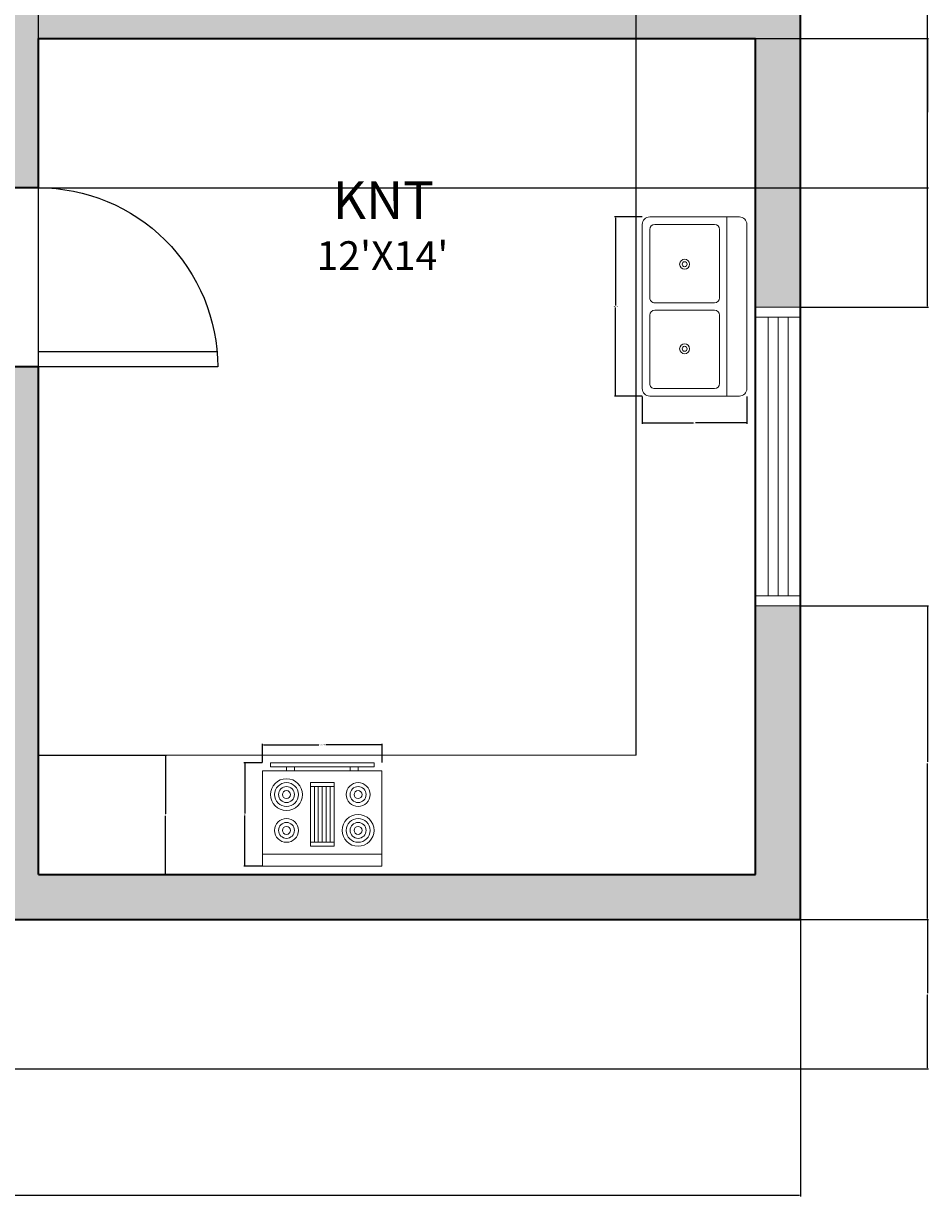
# Model space of a CAD drawing. Units: inches. Extents: x -82 to 330, y 553 to 1115.
# Tile 2 of 4: x 148 to 330, y 553 to 789. Entities that reach past the tile are written whole.
import ezdxf

# ---------------------------------------------------------------- set-up
doc = ezdxf.new("R2010")
doc.units = ezdxf.units.IN
for name, color, linetype, lineweight in [('A-ANNO-DIMS', 2, 'Continuous', 18), ('A-AREA-IDEN', 7, 'Continuous', 25), ('A-DOOR', 3, 'Continuous', 25), ('A-EQPM', 9, 'Continuous', 18), ('A-FLOR-CASE', 8, 'Continuous', 18), ('A-FLOR-FIXT', 8, 'Continuous', 18), ('A-GLAZ', 4, 'Continuous', 18), ('A-WALL', 7, 'Continuous', 35)]:
    doc.layers.add(name, color=color, linetype=linetype, lineweight=lineweight)
doc.layers.add('A-WALL-PATT', color=18, linetype='Continuous', lineweight=13, true_color=0x000000)
doc.styles.get("Standard").update_dxf_attribs({"font": 'arial.ttf'})
doc.dimstyles.get("Standard").update_dxf_attribs({"dimtxt": 0.18, "dimasz": 0.18, "dimexe": 0.18, "dimexo": 0.0625, "dimgap": 0.09, "dimtad": 0, "dimtih": 1, "dimtoh": 1, "dimdec": 4, "dimzin": 0, "dimdsep": 46, "dimtxsty": 'Standard', "dimcen": 0.09, "dimadec": 0, "dimazin": 0, "dimtfac": 1, "dimtdec": 4, "dimtofl": 0, "dimtmove": 0, "dimatfit": 3, "dimfxl": 1, "dimtolj": 1, "dimtzin": 0, "dimarcsym": 0})

# ---------------------------------------------------------------- blocks, each defined once
blk = doc.blocks.new('Sink-double - 36 in top')
for p, q in [((-18, -4), (18, -4)), ((-0.75, -18.5), (-0.75, -6.5)), ((0.75, -6.5), (0.75, -18.5))]:
    blk.add_line(p, q)
for points in [[(-16.5, 0), (16.5, 0)], [(-18, -19.5), (-18, -1.5)], [(18, -1.5), (18, -19.5)], [(-16.5, -18.5), (-16.5, -6.5)], [(-15.5, -5.5), (-1.75, -5.5)], [(1.75, -5.5), (15.5, -5.5)], [(16.5, -6.5), (16.5, -18.5)], [(16.5, -21), (-16.5, -21)], [(-1.75, -19.5), (-15.5, -19.5)], [(15.5, -19.5), (1.75, -19.5)]]:
    blk.add_lwpolyline(points)
for centre, radius in [((-8.5, -12.5), 1), ((8.5, -12.5), 1), ((-8.5, -12.5), 0.5), ((8.5, -12.5), 0.5)]:
    blk.add_circle(centre, radius)
for centre, radius, start, end in [((-16.5, -1.5), 1.5, 90, 180), ((16.5, -1.5), 1.5, 0, 90), ((-15.5, -6.5), 1, 90, 180), ((-1.75, -6.5), 1, 0, 90), ((1.75, -6.5), 1, 90, 180), ((15.5, -6.5), 1, 0, 90), ((-15.5, -18.5), 1, 180, 270), ((-1.75, -18.5), 1, 270, 0), ((1.75, -18.5), 1, 180, 270), ((15.5, -18.5), 1, 270, 0), ((-16.5, -19.5), 1.5, 180, 270), ((16.5, -19.5), 1.5, 270, 0)]:
    blk.add_arc(centre, radius, start, end)
blk = doc.blocks.new('Range-Oven - 30 in top')
for p, q in [((0, -3), (30, -3)), ((12, -6), (18, -6)), ((13, -20), (13, -6)), ((14, -6), (14, -20)), ((15, -20), (15, -6)), ((16, -6), (16, -20)), ((17, -20), (17, -6)), ((18, -20), (12, -20)), ((6, -24), (6, -25)), ((8, -25), (8, -24)), ((22, -25), (22, -24)), ((24, -24), (24, -25))]:
    blk.add_line(p, q)
for points in [[(0, -24), (0, 0), (30, 0), (30, -24)], [(12, -21), (12, -5), (18, -5), (18, -21)], [(2, -26), (2, -25), (28, -25), (28, -26)]]:
    blk.add_lwpolyline(points, close=True)
for centre, radius in [((6, -9), 4), ((6, -9), 3), ((6, -9), 2), ((6, -9), 1), ((24, -9), 3), ((24, -9), 2), ((24, -9), 1), ((24, -18), 4), ((6, -18), 3), ((6, -18), 2), ((6, -18), 1), ((24, -18), 3), ((24, -18), 2), ((24, -18), 1)]:
    blk.add_circle(centre, radius)
blk = doc.blocks.new('WIN-60IN')
for p, q in [((60, 9), (0, 9)), ((0, 9), (0, 0)), ((2, 9), (2, 0)), ((58, 0), (58, 9)), ((60, 0), (60, 9)), ((2, 6.5), (58, 6.5)), ((2, 4.5), (58, 4.5)), ((2, 2.5), (58, 2.5)), ((0, 0), (60, 0))]:
    blk.add_line(p, q)
blk = doc.blocks.new('DOOR-SWING-36IN')
for p, q in [((0, 36), (0, 0)), ((3, 36), (3, 0)), ((0, 0), (3, 0))]:
    blk.add_line(p, q)
blk.add_arc((0, 0), 36, 0, 90)
blk = doc.blocks.new('*D21')
at = {"layer": 'A-ANNO-DIMS', "color": 0, "lineweight": -2, "transparency": 16777216}
for p, q in [((272.17, 750.25), (266.65, 750.25)), ((266.83, 750.07), (266.83, 732.43)), ((266.83, 714.43), (266.83, 732.06)), ((272.17, 714.25), (266.65, 714.25))]:
    blk.add_line(p, q, dxfattribs=at)
at = {"layer": 'A-ANNO-DIMS', "color": 0, "transparency": 16777216}
for points in [[(266.8, 750.07), (266.86, 750.07), (266.83, 750.25)], [(266.8, 714.43), (266.86, 714.43), (266.83, 714.25)]]:
    blk.add_solid(points, dxfattribs=at)
at = {"layer": 'Defpoints', "color": 0, "transparency": 16777216}
for p in [(272.23, 750.25), (266.83, 714.25), (272.23, 714.25)]:
    blk.add_point(p, dxfattribs=at)
at = {"layer": 'A-ANNO-DIMS', "color": 0, "transparency": 16777216, "insert": (266.83, 732.25), "char_height": 0.18, "attachment_point": 5}
blk.add_mtext('\\A1;SINK 36', dxfattribs=at)
blk = doc.blocks.new('*D22')
at = {"layer": 'A-ANNO-DIMS', "color": 0, "lineweight": -2, "transparency": 16777216}
for p, q in [((272.23, 714.18), (272.23, 708.67)), ((293.23, 714.18), (293.23, 708.67)), ((272.41, 708.85), (282.52, 708.85)), ((293.05, 708.85), (282.93, 708.85))]:
    blk.add_line(p, q, dxfattribs=at)
at = {"layer": 'A-ANNO-DIMS', "color": 0, "transparency": 16777216}
for points in [[(272.41, 708.88), (272.41, 708.82), (272.23, 708.85)], [(293.05, 708.88), (293.05, 708.82), (293.23, 708.85)]]:
    blk.add_solid(points, dxfattribs=at)
at = {"layer": 'Defpoints', "color": 0, "transparency": 16777216}
for p in [(272.23, 714.25), (293.23, 714.25), (293.23, 708.85)]:
    blk.add_point(p, dxfattribs=at)
at = {"layer": 'A-ANNO-DIMS', "color": 0, "transparency": 16777216, "insert": (282.73, 708.85), "char_height": 0.18, "attachment_point": 5}
blk.add_mtext('\\A1;21', dxfattribs=at)
blk = doc.blocks.new('*D25')
at = {"layer": 'A-ANNO-DIMS', "color": 0, "lineweight": -2, "transparency": 16777216}
for p, q in [((196, 640.64), (196, 644.35)), ((196.18, 644.17), (207.29, 644.17)), ((219.79, 644.17), (208.68, 644.17)), ((219.97, 640.64), (219.97, 644.35))]:
    blk.add_line(p, q, dxfattribs=at)
at = {"layer": 'A-ANNO-DIMS', "color": 0, "transparency": 16777216}
for points in [[(196.18, 644.2), (196.18, 644.14), (196, 644.17)], [(219.79, 644.2), (219.79, 644.14), (219.97, 644.17)]]:
    blk.add_solid(points, dxfattribs=at)
at = {"layer": 'Defpoints', "color": 0, "transparency": 16777216}
for p in [(196, 644.17), (196, 640.58), (219.97, 640.58)]:
    blk.add_point(p, dxfattribs=at)
at = {"layer": 'A-ANNO-DIMS', "color": 0, "transparency": 16777216, "insert": (207.98, 644.17), "char_height": 0.18, "attachment_point": 5}
blk.add_mtext('\\A1;RANGE 24', dxfattribs=at)
blk = doc.blocks.new('*D26')
at = {"layer": 'A-ANNO-DIMS', "color": 0, "lineweight": -2, "transparency": 16777216}
for p, q in [((195.93, 640.58), (192.22, 640.58)), ((192.4, 640.4), (192.4, 630.37)), ((192.4, 619.98), (192.4, 630.01)), ((195.93, 619.8), (192.22, 619.8))]:
    blk.add_line(p, q, dxfattribs=at)
at = {"layer": 'A-ANNO-DIMS', "color": 0, "transparency": 16777216}
for points in [[(192.37, 640.4), (192.43, 640.4), (192.4, 640.58)], [(192.37, 619.98), (192.43, 619.98), (192.4, 619.8)]]:
    blk.add_solid(points, dxfattribs=at)
at = {"layer": 'Defpoints', "color": 0, "transparency": 16777216}
for p in [(196, 640.58), (192.4, 619.8), (196, 619.8)]:
    blk.add_point(p, dxfattribs=at)
at = {"layer": 'A-ANNO-DIMS', "color": 0, "transparency": 16777216, "insert": (192.4, 630.19), "char_height": 0.18, "attachment_point": 5}
blk.add_mtext('\\A1;21', dxfattribs=at)
blk = doc.blocks.new('*D31')
at = {"layer": 'A-ANNO-DIMS', "color": 0, "lineweight": -2, "transparency": 16777216}
for p, q in [((-56.01, 609.05), (-56.01, 553.43)), ((303.99, 609.05), (303.99, 553.43)), ((-55.83, 553.61), (123.7, 553.61)), ((303.81, 553.61), (124.28, 553.61))]:
    blk.add_line(p, q, dxfattribs=at)
at = {"layer": 'A-ANNO-DIMS', "color": 0, "transparency": 16777216}
for points in [[(-55.83, 553.64), (-55.83, 553.58), (-56.01, 553.61)], [(303.81, 553.64), (303.81, 553.58), (303.99, 553.61)]]:
    blk.add_solid(points, dxfattribs=at)
at = {"layer": 'Defpoints', "color": 0, "transparency": 16777216}
for p in [(-56.01, 609.11), (303.99, 609.11), (303.99, 553.61)]:
    blk.add_point(p, dxfattribs=at)
at = {"layer": 'A-ANNO-DIMS', "color": 0, "transparency": 16777216, "insert": (123.99, 553.61), "char_height": 0.18, "attachment_point": 5}
blk.add_mtext('\\A1;360', dxfattribs=at)
blk = doc.blocks.new('*D37')
at = {"layer": 'A-ANNO-DIMS', "color": 0, "lineweight": -2, "transparency": 16777216}
for p, q in [((85.05, 609.11), (329.67, 609.11)), ((329.49, 608.93), (329.49, 594.29)), ((329.49, 579.29), (329.49, 593.93)), ((85.05, 579.11), (329.67, 579.11))]:
    blk.add_line(p, q, dxfattribs=at)
at = {"layer": 'A-ANNO-DIMS', "color": 0, "transparency": 16777216}
for points in [[(329.46, 608.93), (329.52, 608.93), (329.49, 609.11)], [(329.46, 579.29), (329.52, 579.29), (329.49, 579.11)]]:
    blk.add_solid(points, dxfattribs=at)
at = {"layer": 'Defpoints', "color": 0, "transparency": 16777216}
for p in [(84.99, 609.11), (329.49, 609.11), (84.99, 579.11)]:
    blk.add_point(p, dxfattribs=at)
at = {"layer": 'A-ANNO-DIMS', "color": 0, "transparency": 16777216, "insert": (329.49, 594.11), "char_height": 0.18, "attachment_point": 5}
blk.add_mtext('\\A1;30', dxfattribs=at)
blk = doc.blocks.new('*D38')
at = {"layer": 'A-ANNO-DIMS', "color": 0, "lineweight": -2, "transparency": 16777216}
for p, q in [((304.05, 672.11), (329.67, 672.11)), ((329.49, 671.93), (329.49, 640.79)), ((329.49, 609.29), (329.49, 640.43)), ((304.05, 609.11), (329.67, 609.11))]:
    blk.add_line(p, q, dxfattribs=at)
at = {"layer": 'A-ANNO-DIMS', "color": 0, "transparency": 16777216}
for points in [[(329.46, 671.93), (329.52, 671.93), (329.49, 672.11)], [(329.46, 609.29), (329.52, 609.29), (329.49, 609.11)]]:
    blk.add_solid(points, dxfattribs=at)
at = {"layer": 'Defpoints', "color": 0, "transparency": 16777216}
for p in [(303.99, 672.11), (329.49, 672.11), (303.99, 609.11)]:
    blk.add_point(p, dxfattribs=at)
at = {"layer": 'A-ANNO-DIMS', "color": 0, "transparency": 16777216, "insert": (329.49, 640.61), "char_height": 0.18, "attachment_point": 5}
blk.add_mtext('\\A1;63', dxfattribs=at)
blk = doc.blocks.new('*D39')
at = {"layer": 'A-ANNO-DIMS', "color": 0, "lineweight": -2, "transparency": 16777216}
for p, q in [((304.05, 855.11), (329.67, 855.11)), ((329.49, 854.93), (329.49, 793.79)), ((329.49, 732.29), (329.49, 793.43)), ((304.05, 732.11), (329.67, 732.11))]:
    blk.add_line(p, q, dxfattribs=at)
at = {"layer": 'A-ANNO-DIMS', "color": 0, "transparency": 16777216}
for points in [[(329.46, 854.93), (329.52, 854.93), (329.49, 855.11)], [(329.46, 732.29), (329.52, 732.29), (329.49, 732.11)]]:
    blk.add_solid(points, dxfattribs=at)
at = {"layer": 'Defpoints', "color": 0, "transparency": 16777216}
for p in [(303.99, 855.11), (329.49, 855.11), (303.99, 732.11)]:
    blk.add_point(p, dxfattribs=at)
at = {"layer": 'A-ANNO-DIMS', "color": 0, "transparency": 16777216, "insert": (329.49, 793.61), "char_height": 0.18, "attachment_point": 5}
blk.add_mtext('\\A1;123', dxfattribs=at)
blk = doc.blocks.new('*D44')
at = {"layer": 'A-ANNO-DIMS', "color": 0, "lineweight": -2, "transparency": 16777216}
for p, q in [((151.05, 786.11), (329.67, 786.11)), ((329.49, 785.93), (329.49, 771.29)), ((329.49, 756.29), (329.49, 770.93)), ((151.05, 756.11), (329.67, 756.11))]:
    blk.add_line(p, q, dxfattribs=at)
at = {"layer": 'A-ANNO-DIMS', "color": 0, "transparency": 16777216}
for points in [[(329.46, 785.93), (329.52, 785.93), (329.49, 786.11)], [(329.46, 756.29), (329.52, 756.29), (329.49, 756.11)]]:
    blk.add_solid(points, dxfattribs=at)
at = {"layer": 'Defpoints', "color": 0, "transparency": 16777216}
for p in [(150.99, 786.11), (150.99, 756.11), (329.49, 756.11)]:
    blk.add_point(p, dxfattribs=at)
at = {"layer": 'A-ANNO-DIMS', "color": 0, "transparency": 16777216, "insert": (329.49, 771.11), "char_height": 0.18, "attachment_point": 5}
blk.add_mtext('\\A1;30', dxfattribs=at)
blk = doc.blocks.new('*D49')
at = {"layer": 'A-ANNO-DIMS', "color": 0, "lineweight": -2, "transparency": 16777216}
for p, q in [((150.99, 642.17), (150.99, 1114.79)), ((270.99, 642.17), (270.99, 1114.79)), ((151.17, 1114.61), (210.71, 1114.61)), ((270.81, 1114.61), (211.27, 1114.61))]:
    blk.add_line(p, q, dxfattribs=at)
at = {"layer": 'A-ANNO-DIMS', "color": 0, "transparency": 16777216}
for points in [[(151.17, 1114.64), (151.17, 1114.58), (150.99, 1114.61)], [(270.81, 1114.64), (270.81, 1114.58), (270.99, 1114.61)]]:
    blk.add_solid(points, dxfattribs=at)
at = {"layer": 'Defpoints', "color": 0, "transparency": 16777216}
for p in [(270.99, 1114.61), (150.99, 642.11), (270.99, 642.11)]:
    blk.add_point(p, dxfattribs=at)
at = {"layer": 'A-ANNO-DIMS', "color": 0, "transparency": 16777216, "insert": (210.99, 1114.61), "char_height": 0.18, "attachment_point": 5}
blk.add_mtext('\\A1;120', dxfattribs=at)
blk = doc.blocks.new('*D50')
at = {"layer": 'A-ANNO-DIMS', "color": 0, "lineweight": -2, "transparency": 16777216}
for p, q in [((151.05, 642.11), (176.67, 642.11)), ((176.49, 641.93), (176.49, 630.29)), ((176.49, 618.29), (176.49, 629.93)), ((151.05, 618.11), (176.67, 618.11))]:
    blk.add_line(p, q, dxfattribs=at)
at = {"layer": 'A-ANNO-DIMS', "color": 0, "transparency": 16777216}
for points in [[(176.46, 641.93), (176.52, 641.93), (176.49, 642.11)], [(176.46, 618.29), (176.52, 618.29), (176.49, 618.11)]]:
    blk.add_solid(points, dxfattribs=at)
at = {"layer": 'Defpoints', "color": 0, "transparency": 16777216}
for p in [(150.99, 642.11), (150.99, 618.11), (176.49, 618.11)]:
    blk.add_point(p, dxfattribs=at)
at = {"layer": 'A-ANNO-DIMS', "color": 0, "transparency": 16777216, "insert": (176.49, 630.11), "char_height": 0.18, "attachment_point": 5}
blk.add_mtext('\\A1;24', dxfattribs=at)

msp = doc.modelspace()

# ---------------------------------------------------------------- hatches: boundary and pattern name
at = {"layer": 'A-WALL-PATT'}
h = msp.add_hatch(color=256, dxfattribs=at)
h.dxf.hatch_style = 1
h.paths.add_polyline_path([(6.988, 1089.11), (-56.012, 1089.11), (-56.012, 705.11), (-47.012, 705.11), (-15.012, 705.11), (-15.012, 714.11), (-47.012, 714.11), (-47.012, 930.11), (79.988, 930.11), (79.988, 936.11), (-47.012, 936.11), (-47.012, 1080.11), (6.988, 1080.11)])
h.paths.add_polyline_path([(180.988, 1089.11), (66.988, 1089.11), (66.988, 1080.11), (120.988, 1080.11), (120.988, 936.11), (115.988, 936.11), (115.988, 930.11), (131.988, 930.11), (131.988, 936.11), (126.988, 936.11), (126.988, 1080.11), (180.988, 1080.11)])
h.paths.add_polyline_path([(303.988, 1089.11), (240.988, 1089.11), (240.988, 1080.11), (294.988, 1080.11), (294.988, 936.11), (167.988, 936.11), (167.988, 930.11), (180.988, 930.11), (180.988, 834.11), (186.988, 834.11), (186.988, 930.11), (294.988, 930.11), (294.988, 867.11), (303.988, 867.11)])
h.paths.add_polyline_path([(303.988, 855.11), (294.988, 855.11), (294.988, 792.11), (186.988, 792.11), (186.988, 804.11), (180.988, 804.11), (180.988, 792.11), (144.988, 792.11), (144.988, 756.11), (150.988, 756.11), (150.988, 786.11), (294.988, 786.11), (294.988, 732.11), (303.988, 732.11)])
h.paths.add_polyline_path([(303.988, 672.11), (294.988, 672.11), (294.988, 618.11), (150.988, 618.11), (150.988, 720.11), (144.988, 720.11), (144.988, 714.11), (124.988, 714.11), (124.988, 705.11), (144.988, 705.11), (144.988, 618.11), (144.988, 609.11), (303.988, 609.11)])
h.paths.add_polyline_path([(76.988, 714.11), (44.988, 714.11), (44.988, 705.11), (76.988, 705.11)], flags=17)

# ---------------------------------------------------------------- linework, layer by layer
at = {"layer": 'A-FLOR-CASE'}
for p, q in [((270.988, 642.11), (270.988, 786.11)), ((150.988, 642.11), (270.988, 642.11))]:
    msp.add_line(p, q, dxfattribs=at)
at = {"layer": 'A-WALL'}
for p, q in [((303.988, 609.11), (303.988, 1089.11)), ((150.988, 786.11), (294.988, 786.11)), ((150.988, 756.11), (150.988, 786.11)), ((294.988, 618.11), (294.988, 786.11)), ((150.988, 756.11), (144.988, 756.11)), ((150.988, 720.11), (144.988, 720.11)), ((150.988, 618.11), (150.988, 720.11)), ((150.988, 618.11), (294.988, 618.11)), ((84.988, 609.11), (303.988, 609.11))]:
    msp.add_line(p, q, dxfattribs=at)

# ---------------------------------------------------------------- block references
at = {"layer": 'A-DOOR', "extrusion": (0, 0, -1), "zscale": -1, "rotation": 89.99999999999984}
msp.add_blockref('DOOR-SWING-36IN', (-150.988, 720.11), dxfattribs=at)
at = {"layer": 'A-EQPM', "xscale": 0.7990443305677905, "yscale": 0.7990443305677905, "zscale": 0.7990443305677905, "rotation": 180}
msp.add_blockref('Range-Oven - 30 in top', (219.968, 619.802), dxfattribs=at)
at = {"layer": 'A-FLOR-FIXT', "rotation": 270}
msp.add_blockref('Sink-double - 36 in top', (293.228, 732.246), dxfattribs=at)
at = {"layer": 'A-GLAZ', "rotation": 89.99999999999969}
msp.add_blockref('WIN-60IN', (303.989, 672.11), dxfattribs=at)

# ---------------------------------------------------------------- texts
at = {"layer": 'A-AREA-IDEN', "attachment_point": 1}
for s, width, gutter_width, insert, char_height in [('KNT', 339.91085, 37.836, (210.095, 757.394), 7.5672), ("12'X14'", 260.24271, 28.968, (206.811, 745.356), 5.7936)]:
    msp.add_mtext_dynamic_manual_height_columns(s, width=width, gutter_width=gutter_width, heights=[0], dxfattribs=dict(at, insert=insert, char_height=char_height))

# ---------------------------------------------------------------- dimensions: what is measured, and where the dimension line sits
at = {"layer": 'A-ANNO-DIMS'}
for base, p1, p2, picture, middle in [((270.988, 1114.611), (150.988, 642.11), (270.988, 642.11), '*D49', (210.988, 1114.611)), ((293.228, 708.846), (272.228, 714.246), (293.228, 714.246), '*D22', (282.728, 708.846)), ((303.988, 553.609), (-56.012, 609.11), (303.988, 609.11), '*D31', (123.988, 553.609))]:
    dim = msp.add_linear_dim(base=base, p1=p1, p2=p2, dimstyle='Standard', override={"dimdec": 0, "dimlfac": 1, "dimrnd": 0, "dimzin": 0, "dimdsep": 46, "dimlunit": 2}, dxfattribs=at)
    dim.commit()
    dim.dimension.update_dxf_attribs({"geometry": picture, "text_midpoint": middle})
for base, p1, p2, angle, picture, middle in [((329.489, 855.11), (303.988, 732.11), (303.988, 855.11), 90, '*D39', (329.489, 793.61)), ((329.489, 756.11), (150.988, 786.11), (150.988, 756.11), 90, '*D44', (329.489, 771.11)), ((329.489, 672.11), (303.988, 609.11), (303.988, 672.11), 90, '*D38', (329.489, 640.61)), ((176.489, 618.11), (150.988, 642.11), (150.988, 618.11), 270, '*D50', (176.489, 630.11)), ((192.401, 619.802), (195.996, 640.577), (195.996, 619.802), 270, '*D26', (192.401, 630.19)), ((329.489, 609.11), (84.988, 579.11), (84.988, 609.11), 90, '*D37', (329.489, 594.11))]:
    dim = msp.add_linear_dim(base=base, p1=p1, p2=p2, angle=angle, dimstyle='Standard', override={"dimdec": 0, "dimlfac": 1, "dimrnd": 0, "dimzin": 0, "dimdsep": 46, "dimlunit": 2}, dxfattribs=at)
    dim.commit()
    dim.dimension.update_dxf_attribs({"geometry": picture, "text_midpoint": middle})
for base, p1, p2, angle, text, picture, middle in [((266.828, 714.246), (272.228, 750.246), (272.228, 714.246), 270, 'SINK <>', '*D21', (266.828, 732.246)), ((195.996, 644.173), (219.968, 640.577), (195.996, 640.577), 180, 'RANGE <>', '*D25', (207.982, 644.173))]:
    dim = msp.add_linear_dim(base=base, p1=p1, p2=p2, angle=angle, text=text, dimstyle='Standard', override={"dimdec": 0, "dimlfac": 1, "dimrnd": 0, "dimzin": 0, "dimdsep": 46, "dimlunit": 2}, dxfattribs=at)
    dim.commit()
    dim.dimension.update_dxf_attribs({"geometry": picture, "text_midpoint": middle})

doc.saveas('drawing.dxf')
